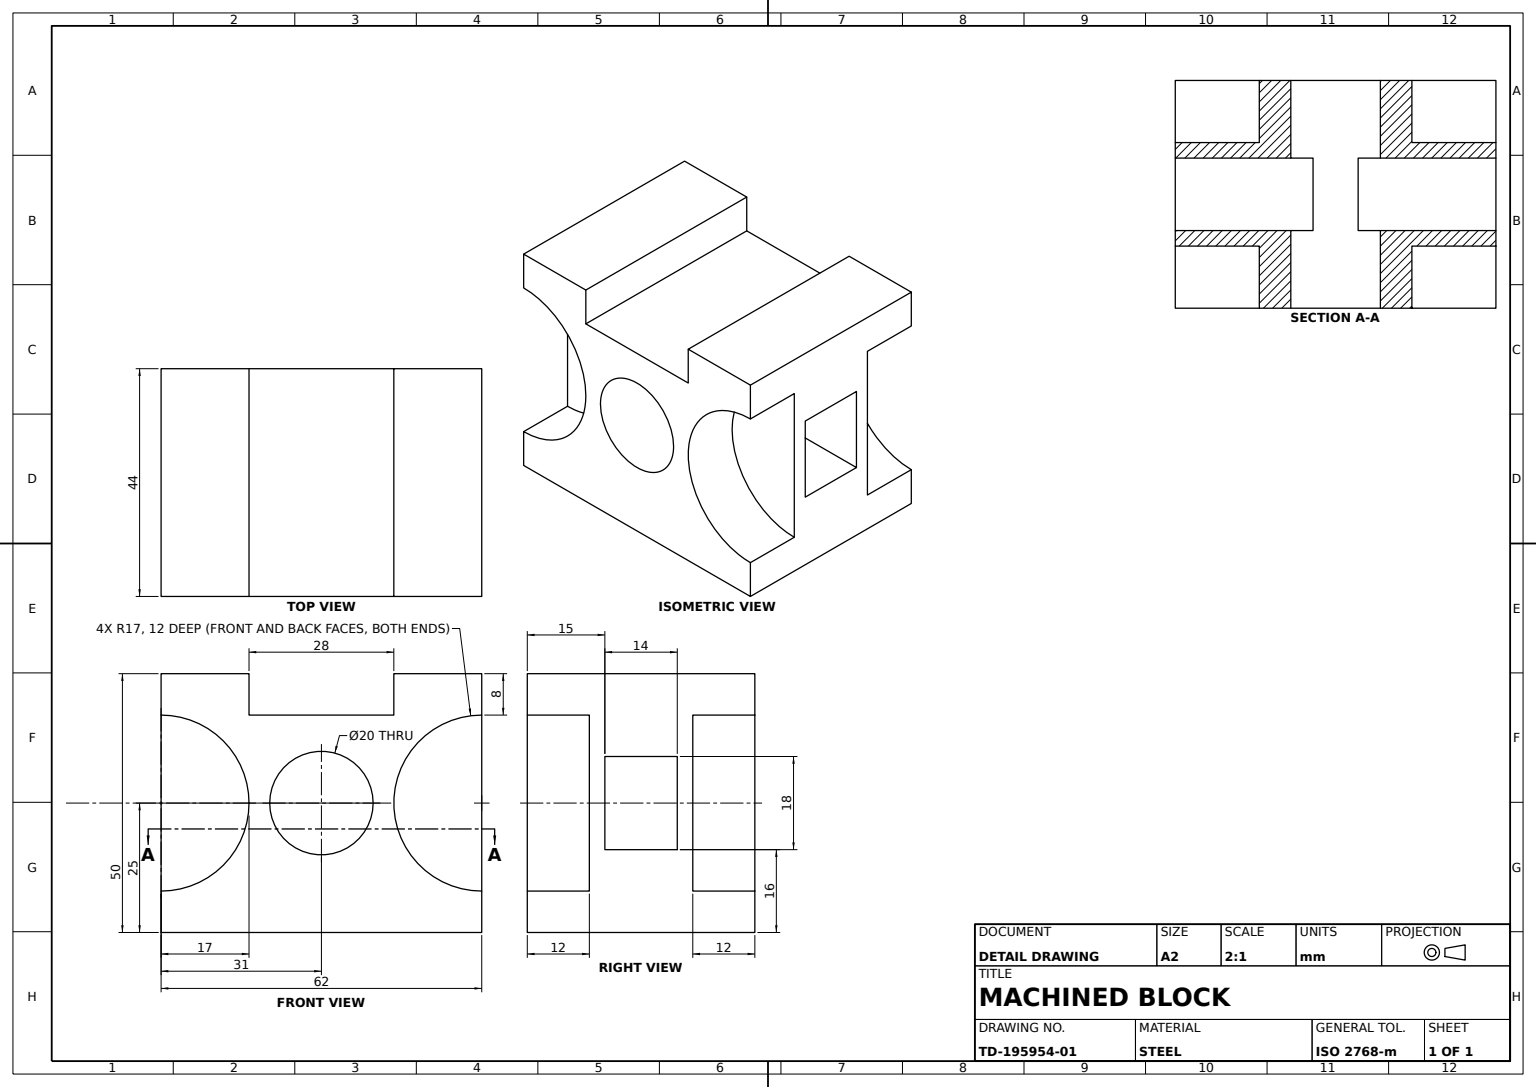
SolidWorks part; units mm, degrees
material "Plain Carbon Steel"
ref_plane "Front Plane" through (0, 0, 0) normal (0, 0, 1) x (1, 0, 0)
ref_plane "Top Plane" through (0, 0, 0) normal (0, 1, 0) x (1, 0, 0)
ref_plane "Right Plane" through (0, 0, 0) normal (1, 0, 0) x (0, 0, -1)
sketch "Block Profile Sketch" plane through (0, 0, 0) normal (0, 0, 1) x (1, 0, 0)
  line L1 (-31, -25) -> (31, -25)
  line L2 (-31, -25) -> (-31, 25)
  line L3 (-31, 25) -> (31, 25)
  line L4 (31, -25) -> (31, 25)
  line L5 (-31, -25) -> (31, 25) construction
  line L6 (-31, 25) -> (31, -25) construction
  point P0 (0, 0)
  dimension "D1" = 50
  dimension "D2" = 62
extrude "Block 62x50x44" add sketch "Block Profile Sketch" along normal blind 44
sketch "Through Hole Sketch" plane through (0, 0, 44) normal (0, 0, 1) x (1, 0, 0)
  circle A0 centre (0, 0) radius 10
  dimension "D1" = 20
extrude "Through Hole Ø20" cut sketch "Through Hole Sketch" against normal blind 44
sketch "Top Slot Sketch" plane through (0, 0, 44) normal (0, 0, 1) x (1, 0, 0)
  line L0 (31, -25) -> (31, 25) construction
  line L1 (31, 17) -> (31, -17)
  arc A0 (31, 17) -> (31, -17) centre (31, 0) ccw
  dimension "D1" = 34
extrude "Top Slot 34x12" cut sketch "Top Slot Sketch" against normal blind 12
sketch "Relief Cut A Sketch" plane through (0, 0, 44) normal (0, 0, 1) x (1, 0, 0)
  line L0 (0, 10) -> (0, -10) construction
  line L1 (31, -17) -> (31, 17)
  line L2 (31, -17) -> (31, 17)
  line L3 (-31, -17) -> (-31, 17)
  circle A0 centre (0, 0) radius 10 construction
  arc A1 (31, 17) -> (31, -17) centre (31, 0) ccw
  arc A2 (31, 17) -> (31, -17) centre (31, 0) ccw
  arc A3 (-31, 17) -> (-31, -17) centre (-31, 0) cw
  dimension "D1" = 0
extrude "Relief Cut A" cut sketch "Relief Cut A Sketch" against normal blind 12
sketch "Side Relief Sketch" plane through (0, 0, 44) normal (0, 0, 1) x (1, 0, 0)
  line L0 (-14, 25) -> (-14, 17)
  line L1 (31, 25) -> (-31, 25) construction
  line L2 (-14, 17) -> (14, 17)
  line L3 (14, 17) -> (14, 25)
  dimension "D1" = 28
  dimension "D2" = 8
  dimension "D3" = 17
extrude "Side Relief Cut" cut sketch "Side Relief Sketch" against normal through all and the other way through all
sketch "Relief Cut B Sketch" plane through (0, 0, 0) normal (0, 0, -1) x (-1, 0, 0)
  line L1 (31, -17) -> (31, 17)
  line L2 (31, -17) -> (31, 17)
  line L8 (31, 25) -> (14, 25)
  line L9 (14, 25) -> (14, 17)
  line L10 (14, 17) -> (-14, 17)
  line L11 (-14, 17) -> (-14, 25)
  line L12 (-14, 25) -> (-31, 25)
  line L13 (-31, 25) -> (-31, -25)
  line L14 (-31, -25) -> (31, -25)
  line L15 (31, -25) -> (31, 25)
  line L16 (31, 25) -> (14, 25)
  line L17 (14, 25) -> (14, 17)
  line L18 (14, 17) -> (-14, 17)
  line L19 (-14, 17) -> (-14, 25)
  line L20 (-14, 25) -> (-31, 25)
  line L21 (-31, 25) -> (-31, -25)
  line L22 (-31, -25) -> (31, -25)
  line L23 (31, -25) -> (31, 25)
  arc A1 (31, 17) -> (31, -17) centre (31, 0) ccw
  arc A2 (31, 17) -> (31, -17) centre (31, 0) ccw
  line M19 (31, -25) -> (31, 25)
  dimension "D1" = 0
  dimension "D2" = 0
extrude "Relief Cut B" cut sketch "Relief Cut B Sketch" against normal blind 12 contours A2 M19
sketch "Relief Cut C Sketch" plane through (0, 0, 0) normal (0, 0, -1) x (-1, 0, 0)
  line L1 (-31, 17) -> (-31, -17)
  line L2 (-31, 17) -> (-31, -17)
  line L9 (31, 17) -> (31, 25)
  line L10 (31, 25) -> (14, 25)
  line L11 (14, 25) -> (14, 17)
  line L12 (14, 17) -> (-14, 17)
  line L13 (-14, 17) -> (-14, 25)
  line L14 (-14, 25) -> (-31, 25)
  line L15 (-31, 25) -> (-31, -25)
  line L16 (-31, -25) -> (31, -25)
  line L17 (31, -25) -> (31, -17)
  line L18 (31, 17) -> (31, 25)
  line L19 (31, 25) -> (14, 25)
  line L20 (14, 25) -> (14, 17)
  line L21 (14, 17) -> (-14, 17)
  line L22 (-14, 17) -> (-14, 25)
  line L23 (-14, 25) -> (-31, 25)
  line L24 (-31, 25) -> (-31, -25)
  line L25 (-31, -25) -> (31, -25)
  line L26 (31, -25) -> (31, -17)
  arc A1 (31, 17) -> (31, -17) centre (31, 0) ccw
  arc A2 (31, 17) -> (31, -17) centre (31, 0) ccw
  arc A3 (-31, -17) -> (-31, 17) centre (-31, 0) ccw
  arc A4 (-31, -17) -> (-31, 17) centre (-31, 0) ccw
  line M20 (-31, 25) -> (-31, -25)
  dimension "D1" = 0
  dimension "D2" = 0
extrude "Relief Cut C" cut sketch "Relief Cut C Sketch" against normal blind 12 contours A4 M20
sketch "Window Sketch" plane through (-31, 0, 0) normal (-1, 0, 0) x (0, 0, 1)
  line L0 (44, -25) -> (0, -25) construction
  line L1 (15, 9) -> (29, 9)
  line L2 (15, 9) -> (15, -9)
  line L3 (15, -9) -> (29, -9)
  line L4 (29, 9) -> (29, -9)
  line L5 (15, 9) -> (29, -9) construction
  line L6 (15, -9) -> (29, 9) construction
  line L7 (0, 17) -> (0, -17) construction
  point P0 (22, 0)
  dimension "D1" = 14
  dimension "D2" = 18
  dimension "D3" = 16
  dimension "D4" = 15
extrude "Window Cut" cut sketch "Window Sketch" against normal through all
